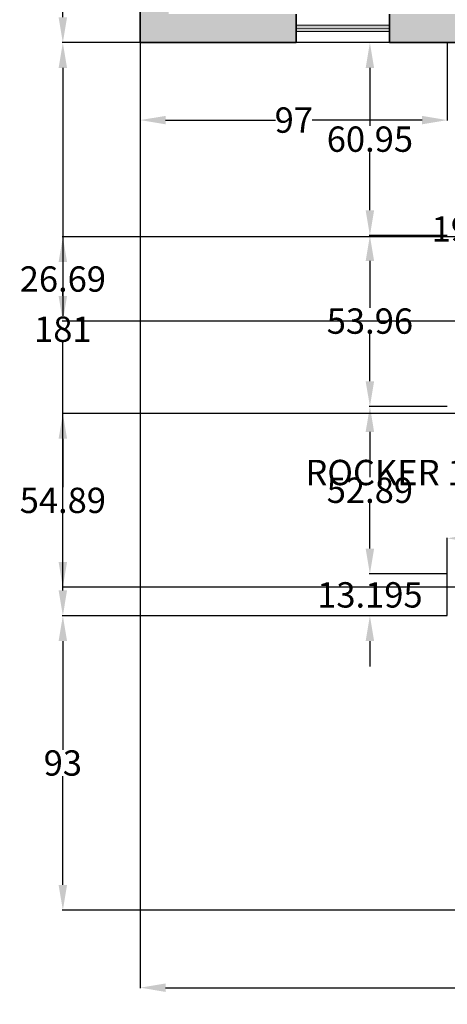
# Model space of a CAD drawing. Units: inches. Extents: x -52 to 678, y 23 to 685.
# Tile 1 of 11: x 54 to 189, y 23 to 334. Entities that reach past the tile are written whole.
import ezdxf

# ---------------------------------------------------------------- set-up
doc = ezdxf.new("R2010")
doc.units = ezdxf.units.IN
doc.header["$MEASUREMENT"] = 0
for name, color, linetype, lineweight in [('A-ANNO-DIMS', 2, 'Continuous', 18), ('A-GLAZ', 4, 'Continuous', 18), ('A-WALL', 7, 'Continuous', 35)]:
    doc.layers.add(name, color=color, linetype=linetype, lineweight=lineweight)
doc.layers.add('A-GLAZ-PATT', color=18, linetype='Continuous', lineweight=13, true_color=0x000000)
doc.layers.add('A-WALL-PATT', color=18, linetype='Continuous', lineweight=13, true_color=0x000000)
doc.styles.get("Standard").update_dxf_attribs({"font": 'arial.ttf'})
doc.dimstyles.get("Standard").update_dxf_attribs({"dimtxt": 8, "dimasz": 8, "dimexe": 0.18, "dimexo": 0.0625, "dimgap": 0.09, "dimtad": 0, "dimtih": 1, "dimtoh": 1, "dimdec": 0, "dimzin": 0, "dimdsep": 46, "dimlunit": 3, "dimtxsty": 'Standard', "dimcen": 0.09, "dimadec": 0, "dimazin": 0, "dimtfac": 1, "dimtdec": 0, "dimtofl": 0, "dimtmove": 0, "dimatfit": 3, "dimfxl": 1, "dimtolj": 1, "dimtzin": 0, "dimarcsym": 0})

# ---------------------------------------------------------------- blocks, each defined once
blk = doc.blocks.new('*D21')
at = {"layer": 'A-ANNO-DIMS', "color": 0, "lineweight": -2, "transparency": 16777216}
for p, q in [((230.65, 223.62), (234.77, 230.48)), ((228.24, 215.74), (226.38, 216.85)), ((221.23, 204.07), (219.38, 205.18)), ((215.42, 198.23), (211.3, 191.37)), ((211.3, 191.37), (203.3, 191.37))]:
    blk.add_line(p, q, dxfattribs=at)
at = {"layer": 'A-ANNO-DIMS', "color": 0, "transparency": 16777216}
for points in [[(229.51, 224.3), (231.8, 222.93), (226.54, 216.76)], [(214.28, 198.91), (216.56, 197.54), (219.54, 205.09)]]:
    blk.add_solid(points, dxfattribs=at)
at = {"layer": 'Defpoints', "color": 0, "transparency": 16777216}
for p in [(228.29, 215.71), (219.54, 205.09), (221.29, 204.04)]:
    blk.add_point(p, dxfattribs=at)
at = {"layer": 'A-ANNO-DIMS', "color": 0, "transparency": 16777216, "insert": (172.25, 191.37), "char_height": 8, "attachment_point": 5}
blk.add_mtext('\\A1;ROCKER 14', dxfattribs=at)
blk = doc.blocks.new('*D26')
at = {"layer": 'A-ANNO-DIMS', "color": 0, "lineweight": -2, "transparency": 16777216}
for p, q in [((203.16, 268.27), (195.16, 268.27)), ((203.16, 261.94), (203.16, 268.45)), ((213.77, 268.27), (211.16, 268.27)), ((221.77, 261.94), (221.77, 268.45))]:
    blk.add_line(p, q, dxfattribs=at)
at = {"layer": 'A-ANNO-DIMS', "color": 0, "transparency": 16777216}
for points in [[(211.16, 269.61), (211.16, 266.94), (203.16, 268.27)], [(213.77, 269.61), (213.77, 266.94), (221.77, 268.27)]]:
    blk.add_solid(points, dxfattribs=at)
at = {"layer": 'Defpoints', "color": 0, "transparency": 16777216}
for p in [(203.16, 268.27), (203.16, 261.88), (221.77, 261.88)]:
    blk.add_point(p, dxfattribs=at)
at = {"layer": 'A-ANNO-DIMS', "color": 0, "transparency": 16777216, "insert": (189.71, 268.27), "char_height": 8, "attachment_point": 5}
blk.add_mtext('\\A1;19', dxfattribs=at)
blk = doc.blocks.new('*D39')
at = {"layer": 'A-ANNO-DIMS', "color": 0, "lineweight": -2, "transparency": 16777216}
for p, q in [((91.61, 327.06), (91.61, 28.49)), ((575.61, 53.06), (575.61, 28.49)), ((99.61, 28.67), (324.53, 28.67)), ((567.61, 28.67), (342.68, 28.67))]:
    blk.add_line(p, q, dxfattribs=at)
at = {"layer": 'A-ANNO-DIMS', "color": 0, "transparency": 16777216}
for points in [[(99.61, 30), (99.61, 27.33), (91.61, 28.67)], [(567.61, 30), (567.61, 27.33), (575.61, 28.67)]]:
    blk.add_solid(points, dxfattribs=at)
at = {"layer": 'Defpoints', "color": 0, "transparency": 16777216}
for p in [(91.61, 327.13), (575.61, 53.13), (575.61, 28.67)]:
    blk.add_point(p, dxfattribs=at)
at = {"layer": 'A-ANNO-DIMS', "color": 0, "transparency": 16777216, "insert": (333.61, 28.67), "char_height": 8, "attachment_point": 5}
blk.add_mtext('\\A1;484', dxfattribs=at)
blk = doc.blocks.new('*D45')
at = {"layer": 'A-ANNO-DIMS', "color": 0, "lineweight": -2, "transparency": 16777216}
for p, q in [((91.54, 477.13), (66.97, 477.13)), ((67.15, 469.13), (67.15, 406.3)), ((67.15, 335.13), (67.15, 397.95)), ((91.54, 327.13), (66.97, 327.13))]:
    blk.add_line(p, q, dxfattribs=at)
at = {"layer": 'A-ANNO-DIMS', "color": 0, "transparency": 16777216}
for points in [[(65.81, 469.13), (68.48, 469.13), (67.15, 477.13)], [(65.81, 335.13), (68.48, 335.13), (67.15, 327.13)]]:
    blk.add_solid(points, dxfattribs=at)
at = {"layer": 'Defpoints', "color": 0, "transparency": 16777216}
for p in [(67.15, 477.13), (91.61, 477.13), (91.61, 327.13)]:
    blk.add_point(p, dxfattribs=at)
at = {"layer": 'A-ANNO-DIMS', "color": 0, "transparency": 16777216, "insert": (67.15, 402.13), "char_height": 8, "attachment_point": 5}
blk.add_mtext('\\A1;150', dxfattribs=at)
blk = doc.blocks.new('*D46')
at = {"layer": 'A-ANNO-DIMS', "color": 0, "lineweight": -2, "transparency": 16777216}
for p, q in [((188.54, 327.13), (66.97, 327.13)), ((67.15, 319.13), (67.15, 240.8)), ((67.15, 154.13), (67.15, 232.45)), ((188.54, 146.13), (66.97, 146.13))]:
    blk.add_line(p, q, dxfattribs=at)
at = {"layer": 'A-ANNO-DIMS', "color": 0, "transparency": 16777216}
for points in [[(65.81, 319.13), (68.48, 319.13), (67.15, 327.13)], [(65.81, 154.13), (68.48, 154.13), (67.15, 146.13)]]:
    blk.add_solid(points, dxfattribs=at)
at = {"layer": 'Defpoints', "color": 0, "transparency": 16777216}
for p in [(67.15, 327.13), (188.61, 327.13), (188.61, 146.13)]:
    blk.add_point(p, dxfattribs=at)
at = {"layer": 'A-ANNO-DIMS', "color": 0, "transparency": 16777216, "insert": (67.15, 236.63), "char_height": 8, "attachment_point": 5}
blk.add_mtext('\\A1;181', dxfattribs=at)
blk = doc.blocks.new('*D47')
at = {"layer": 'A-ANNO-DIMS', "color": 0, "lineweight": -2, "transparency": 16777216}
for p, q in [((188.54, 146.13), (66.97, 146.13)), ((67.15, 138.13), (67.15, 103.8)), ((67.15, 61.13), (67.15, 95.45)), ((425.54, 53.13), (66.97, 53.13))]:
    blk.add_line(p, q, dxfattribs=at)
at = {"layer": 'A-ANNO-DIMS', "color": 0, "transparency": 16777216}
for points in [[(65.81, 138.13), (68.48, 138.13), (67.15, 146.13)], [(65.81, 61.13), (68.48, 61.13), (67.15, 53.13)]]:
    blk.add_solid(points, dxfattribs=at)
at = {"layer": 'Defpoints', "color": 0, "transparency": 16777216}
for p in [(67.15, 146.13), (188.61, 146.13), (425.61, 53.13)]:
    blk.add_point(p, dxfattribs=at)
at = {"layer": 'A-ANNO-DIMS', "color": 0, "transparency": 16777216, "insert": (67.15, 99.63), "char_height": 8, "attachment_point": 5}
blk.add_mtext('\\A1;93', dxfattribs=at)
blk = doc.blocks.new('*D48')
at = {"layer": 'A-ANNO-DIMS', "color": 0, "lineweight": -2, "transparency": 16777216}
for p, q in [((91.61, 327.06), (91.61, 302.49)), ((188.61, 327.06), (188.61, 302.49)), ((99.61, 302.67), (134.29, 302.67)), ((180.61, 302.67), (145.93, 302.67))]:
    blk.add_line(p, q, dxfattribs=at)
at = {"layer": 'A-ANNO-DIMS', "color": 0, "transparency": 16777216}
for points in [[(99.61, 304), (99.61, 301.33), (91.61, 302.67)], [(180.61, 304), (180.61, 301.33), (188.61, 302.67)]]:
    blk.add_solid(points, dxfattribs=at)
at = {"layer": 'Defpoints', "color": 0, "transparency": 16777216}
for p in [(91.61, 327.13), (188.61, 327.13), (91.61, 302.67)]:
    blk.add_point(p, dxfattribs=at)
at = {"layer": 'A-ANNO-DIMS', "color": 0, "transparency": 16777216, "insert": (140.11, 302.67), "char_height": 8, "attachment_point": 5}
blk.add_mtext('\\A1;97', dxfattribs=at)
blk = doc.blocks.new('*D49')
at = {"layer": 'A-ANNO-DIMS', "color": 0, "lineweight": -2, "transparency": 16777216}
for p, q in [((188.61, 146.19), (188.61, 170.77)), ((196.61, 170.59), (232.28, 170.59)), ((279.61, 170.59), (243.93, 170.59)), ((287.61, 146.19), (287.61, 170.77))]:
    blk.add_line(p, q, dxfattribs=at)
at = {"layer": 'A-ANNO-DIMS', "color": 0, "transparency": 16777216}
for points in [[(196.61, 171.92), (196.61, 169.25), (188.61, 170.59)], [(279.61, 171.92), (279.61, 169.25), (287.61, 170.59)]]:
    blk.add_solid(points, dxfattribs=at)
at = {"layer": 'Defpoints', "color": 0, "transparency": 16777216}
for p in [(287.61, 170.59), (188.61, 146.13), (287.61, 146.13)]:
    blk.add_point(p, dxfattribs=at)
at = {"layer": 'A-ANNO-DIMS', "color": 0, "transparency": 16777216, "insert": (238.11, 170.59), "char_height": 8, "attachment_point": 5}
blk.add_mtext('\\A1;99', dxfattribs=at)
blk = doc.blocks.new('*D74')
at = {"layer": 'A-ANNO-DIMS', "color": 0, "lineweight": -2, "transparency": 16777216}
for p, q in [((164.15, 167.32), (164.15, 175.32)), ((188.54, 159.32), (163.97, 159.32)), ((188.54, 146.13), (163.97, 146.13)), ((164.15, 138.13), (164.15, 130.13))]:
    blk.add_line(p, q, dxfattribs=at)
at = {"layer": 'A-ANNO-DIMS', "color": 0, "transparency": 16777216}
for points in [[(162.81, 167.32), (165.48, 167.32), (164.15, 159.32)], [(162.81, 138.13), (165.48, 138.13), (164.15, 146.13)]]:
    blk.add_solid(points, dxfattribs=at)
at = {"layer": 'Defpoints', "color": 0, "transparency": 16777216}
for p in [(164.15, 159.32), (188.61, 159.32), (188.61, 146.13)]:
    blk.add_point(p, dxfattribs=at)
at = {"layer": 'A-ANNO-DIMS', "color": 0, "transparency": 16777216, "insert": (164.15, 152.72), "char_height": 8, "attachment_point": 5}
blk.add_mtext('\\A1;13.195', dxfattribs=at)
blk = doc.blocks.new('*D75')
at = {"layer": 'A-ANNO-DIMS', "color": 0, "lineweight": -2, "transparency": 16777216}
for p, q in [((188.54, 212.21), (163.97, 212.21)), ((164.15, 204.21), (164.15, 189.94)), ((164.15, 167.32), (164.15, 181.59)), ((188.54, 159.32), (163.97, 159.32))]:
    blk.add_line(p, q, dxfattribs=at)
at = {"layer": 'A-ANNO-DIMS', "color": 0, "transparency": 16777216}
for points in [[(162.81, 204.21), (165.48, 204.21), (164.15, 212.21)], [(162.81, 167.32), (165.48, 167.32), (164.15, 159.32)]]:
    blk.add_solid(points, dxfattribs=at)
at = {"layer": 'Defpoints', "color": 0, "transparency": 16777216}
for p in [(164.15, 212.21), (188.61, 212.21), (188.61, 159.32)]:
    blk.add_point(p, dxfattribs=at)
at = {"layer": 'A-ANNO-DIMS', "color": 0, "transparency": 16777216, "insert": (164.15, 185.77), "char_height": 8, "attachment_point": 5}
blk.add_mtext('\\A1;52.89', dxfattribs=at)
blk = doc.blocks.new('*D76')
at = {"layer": 'A-ANNO-DIMS', "color": 0, "lineweight": -2, "transparency": 16777216}
for p, q in [((188.54, 266.17), (163.97, 266.17)), ((164.15, 258.17), (164.15, 243.37)), ((164.15, 220.21), (164.15, 235.02)), ((188.54, 212.21), (163.97, 212.21))]:
    blk.add_line(p, q, dxfattribs=at)
at = {"layer": 'A-ANNO-DIMS', "color": 0, "transparency": 16777216}
for points in [[(162.81, 258.17), (165.48, 258.17), (164.15, 266.17)], [(162.81, 220.21), (165.48, 220.21), (164.15, 212.21)]]:
    blk.add_solid(points, dxfattribs=at)
at = {"layer": 'Defpoints', "color": 0, "transparency": 16777216}
for p in [(164.15, 266.17), (188.61, 266.17), (188.61, 212.21)]:
    blk.add_point(p, dxfattribs=at)
at = {"layer": 'A-ANNO-DIMS', "color": 0, "transparency": 16777216, "insert": (164.15, 239.19), "char_height": 8, "attachment_point": 5}
blk.add_mtext('\\A1;53.96', dxfattribs=at)
blk = doc.blocks.new('*D77')
at = {"layer": 'A-ANNO-DIMS', "color": 0, "lineweight": -2, "transparency": 16777216}
for p, q in [((188.54, 327.13), (163.97, 327.13)), ((164.15, 319.13), (164.15, 300.82)), ((164.15, 274.17), (164.15, 292.48)), ((188.54, 266.17), (163.97, 266.17))]:
    blk.add_line(p, q, dxfattribs=at)
at = {"layer": 'A-ANNO-DIMS', "color": 0, "transparency": 16777216}
for points in [[(162.81, 319.13), (165.48, 319.13), (164.15, 327.13)], [(162.81, 274.17), (165.48, 274.17), (164.15, 266.17)]]:
    blk.add_solid(points, dxfattribs=at)
at = {"layer": 'Defpoints', "color": 0, "transparency": 16777216}
for p in [(164.15, 327.13), (188.61, 327.13), (188.61, 266.17)]:
    blk.add_point(p, dxfattribs=at)
at = {"layer": 'A-ANNO-DIMS', "color": 0, "transparency": 16777216, "insert": (164.15, 296.65), "char_height": 8, "attachment_point": 5}
blk.add_mtext('\\A1;60.95', dxfattribs=at)
blk = doc.blocks.new('*D100')
at = {"layer": 'A-ANNO-DIMS', "color": 0, "lineweight": -2, "transparency": 16777216}
for p, q in [((519.99, 265.81), (66.97, 265.81)), ((67.15, 257.81), (67.15, 256.65)), ((67.15, 247.13), (67.15, 248.3)), ((521.98, 239.13), (66.97, 239.13))]:
    blk.add_line(p, q, dxfattribs=at)
at = {"layer": 'A-ANNO-DIMS', "color": 0, "transparency": 16777216}
for points in [[(65.81, 257.81), (68.48, 257.81), (67.15, 265.81)], [(65.81, 247.13), (68.48, 247.13), (67.15, 239.13)]]:
    blk.add_solid(points, dxfattribs=at)
at = {"layer": 'Defpoints', "color": 0, "transparency": 16777216}
for p in [(520.05, 265.81), (67.15, 239.13), (522.04, 239.13)]:
    blk.add_point(p, dxfattribs=at)
at = {"layer": 'A-ANNO-DIMS', "color": 0, "transparency": 16777216, "insert": (67.15, 252.47), "char_height": 8, "attachment_point": 5}
blk.add_mtext('\\A1;26.69', dxfattribs=at)
blk = doc.blocks.new('*D104')
at = {"layer": 'A-ANNO-DIMS', "color": 0, "lineweight": -2, "transparency": 16777216}
for p, q in [((265.91, 210.01), (66.97, 210.01)), ((67.15, 202.01), (67.15, 186.74)), ((67.15, 163.13), (67.15, 178.39)), ((301.21, 155.13), (66.97, 155.13))]:
    blk.add_line(p, q, dxfattribs=at)
at = {"layer": 'A-ANNO-DIMS', "color": 0, "transparency": 16777216}
for points in [[(65.81, 202.01), (68.48, 202.01), (67.15, 210.01)], [(65.81, 163.13), (68.48, 163.13), (67.15, 155.13)]]:
    blk.add_solid(points, dxfattribs=at)
at = {"layer": 'Defpoints', "color": 0, "transparency": 16777216}
for p in [(265.98, 210.01), (67.15, 155.13), (301.27, 155.13)]:
    blk.add_point(p, dxfattribs=at)
at = {"layer": 'A-ANNO-DIMS', "color": 0, "transparency": 16777216, "insert": (67.15, 182.57), "char_height": 8, "attachment_point": 5}
blk.add_mtext('\\A1;54.89', dxfattribs=at)

msp = doc.modelspace()

# ---------------------------------------------------------------- hatches: boundary and pattern name
at = {"layer": 'A-GLAZ-PATT'}
h = msp.add_hatch(color=256, dxfattribs=at)
h.dxf.hatch_style = 1
h.paths.add_polyline_path([(140.8548, 332.6922), (140.8548, 331.6922), (170.301, 331.6267), (170.301, 332.6267)])
h = msp.add_hatch(color=256, dxfattribs=at)
h.dxf.hatch_style = 1
h.paths.add_polyline_path([(170.301, 330.6267), (170.301, 331.6267), (140.8548, 331.6922), (140.8548, 330.6922)])
at = {"layer": 'A-WALL-PATT'}
h = msp.add_hatch(color=256, dxfattribs=at)
h.dxf.hatch_style = 1
h.paths.add_polyline_path([(100.6053, 336.1267), (100.6053, 468.1267), (159.5302, 468.1267), (159.5302, 477.1267), (91.6053, 477.1267), (91.6053, 327.1267), (140.8548, 327.1267), (140.8548, 336.1267), (137.7032, 336.1267)])
h = msp.add_hatch(color=256, dxfattribs=at)
h.dxf.hatch_style = 1
h.paths.add_polyline_path([(265.6053, 327.1267), (265.6053, 336.1267), (170.301, 336.1267), (170.301, 327.1267)])

# ---------------------------------------------------------------- linework, layer by layer
at = {"layer": 'A-GLAZ'}
for p, q in [((140.8525, 330.6922), (170.2987, 330.6267)), ((140.8548, 331.6922), (170.301, 331.6267)), ((140.857, 332.6922), (170.3032, 332.6267)), ((140.8446, 327.1268), (170.2908, 327.0613))]:
    msp.add_line(p, q, dxfattribs=at)
at = {"layer": 'A-WALL'}
for p, q in [((91.6053, 477.1267), (91.6053, 327.1267)), ((140.8548, 336.1267), (140.8548, 327.1267)), ((170.301, 327.1267), (170.301, 336.1267)), ((91.6053, 327.1267), (140.8548, 327.1267)), ((170.301, 327.1267), (265.6053, 327.1267))]:
    msp.add_line(p, q, dxfattribs=at)

# ---------------------------------------------------------------- dimensions: what is measured, and where the dimension line sits
at = {"layer": 'A-ANNO-DIMS'}
for base, p1, p2, angle, override, picture, middle in [((67.1453, 477.1267), (91.6053, 327.1267), (91.6053, 477.1267), 90, {"dimdec": 0, "dimlfac": 1, "dimrnd": 0, "dimzin": 0, "dimdsep": 46, "dimlunit": 2}, '*D45', (67.1453, 402.1267)), ((67.1453, 327.1267), (188.6053, 146.1267), (188.6053, 327.1267), 90, {"dimdec": 0, "dimlfac": 1, "dimrnd": 0, "dimzin": 0, "dimdsep": 46, "dimlunit": 2}, '*D46', (67.1453, 236.6267)), ((91.6053, 302.6667), (188.6053, 327.1267), (91.6053, 327.1267), 180, {"dimdec": 0, "dimlfac": 1, "dimrnd": 0, "dimzin": 0, "dimdsep": 46, "dimlunit": 2}, '*D48', (140.1053, 302.6667)), ((164.1453, 327.1267), (188.6053, 266.1726), (188.6053, 327.1267), 90, {"dimdec": 2, "dimlfac": 1, "dimrnd": 0, "dimzin": 0, "dimdsep": 46, "dimlunit": 2}, '*D77', (164.1453, 296.6497)), ((203.1594, 268.2744), (221.7669, 261.8802), (203.1594, 261.8802), 180, {"dimdec": 0, "dimlfac": 1, "dimrnd": 0, "dimzin": 0, "dimdsep": 46, "dimlunit": 2}, '*D26', (189.7079, 268.2744)), ((67.1453, 239.1267), (520.0511, 265.8145), (522.0448, 239.1267), 90, {"dimdec": 2, "dimlfac": 1, "dimrnd": 0, "dimzin": 0, "dimdsep": 46, "dimlunit": 2}, '*D100', (67.1453, 252.4706)), ((164.1453, 266.1726), (188.6053, 212.2126), (188.6053, 266.1726), 90, {"dimdec": 2, "dimlfac": 1, "dimrnd": 0, "dimzin": 0, "dimdsep": 46, "dimlunit": 2}, '*D76', (164.1453, 239.1926)), ((164.1453, 212.2126), (188.6053, 159.3213), (188.6053, 212.2126), 90, {"dimdec": 2, "dimlfac": 1, "dimrnd": 0, "dimzin": 0, "dimdsep": 46, "dimlunit": 2}, '*D75', (164.1453, 185.767)), ((67.1453, 155.1267), (265.9763, 210.0118), (301.2728, 155.1267), 90, {"dimdec": 2, "dimlfac": 1, "dimrnd": 0, "dimzin": 0, "dimdsep": 46, "dimlunit": 2}, '*D104', (67.1453, 182.5693)), ((164.1453, 159.3213), (188.6053, 146.1267), (188.6053, 159.3213), 90, {"dimdec": 3, "dimlfac": 1, "dimrnd": 0, "dimzin": 0, "dimdsep": 46, "dimlunit": 2}, '*D74', (164.1453, 152.724)), ((67.1453, 146.1267), (425.6053, 53.1267), (188.6053, 146.1267), 90, {"dimdec": 0, "dimlfac": 1, "dimrnd": 0, "dimzin": 0, "dimdsep": 46, "dimlunit": 2}, '*D47', (67.1453, 99.6267))]:
    dim = msp.add_linear_dim(base=base, p1=p1, p2=p2, angle=angle, dimstyle='Standard', override=override, dxfattribs=at)
    dim.commit()
    dim.dimension.update_dxf_attribs({"geometry": picture, "text_midpoint": middle})
for base, p1, p2, picture, middle in [((575.6053, 28.6667), (91.6053, 327.1267), (575.6053, 53.1267), '*D39', (333.6053, 28.6667)), ((287.6053, 170.5867), (188.6053, 146.1267), (287.6053, 146.1267), '*D49', (238.1053, 170.5867))]:
    dim = msp.add_linear_dim(base=base, p1=p1, p2=p2, dimstyle='Standard', override={"dimdec": 0, "dimlfac": 1, "dimrnd": 0, "dimzin": 0, "dimdsep": 46, "dimlunit": 2}, dxfattribs=at)
    dim.commit()
    dim.dimension.update_dxf_attribs({"geometry": picture, "text_midpoint": middle})
dim = msp.add_linear_dim(base=(219.5361, 205.0862), p1=(228.2887, 215.706), p2=(221.2866, 204.0359), angle=239.036213, text='ROCKER <>', dimstyle='Standard', override={"dimdec": 0, "dimlfac": 1, "dimrnd": 0, "dimzin": 0, "dimdsep": 46, "dimlunit": 2}, dxfattribs=at)
dim.commit()
dim.dimension.update_dxf_attribs({"geometry": '*D21', "text_midpoint": (172.2483, 191.3664)})

doc.saveas('drawing.dxf')
